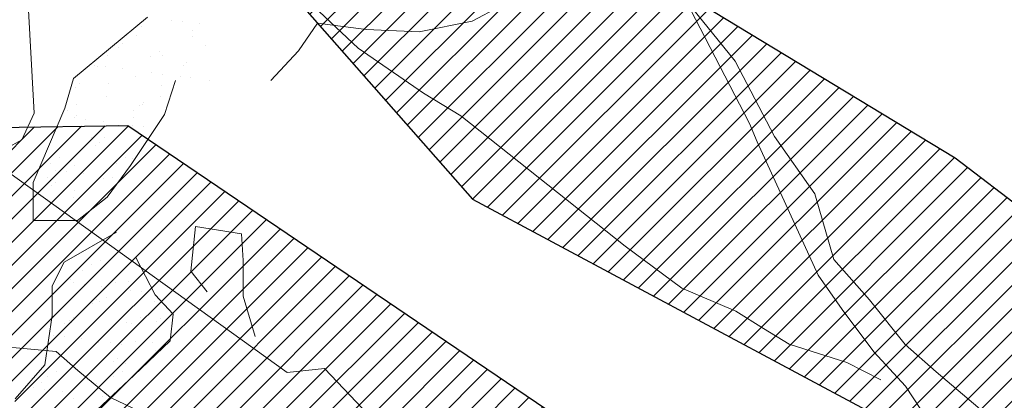
# Model space of a CAD drawing. Units: inches. Extents: x 1986 to 21484, y -1816 to 2016.
# Tile 21 of 85: x 2157.681 to 2166.915, y 1888.377 to 1891.95. Entities that reach past the tile are written whole.
import ezdxf

# ---------------------------------------------------------------- set-up
doc = ezdxf.new("R2010")
doc.units = ezdxf.units.IN
doc.layers.add('L-PLNT', color=84, linetype='Continuous', lineweight=13)
doc.layers.add('vfolhas', color=114, linetype='Continuous', lineweight=5)
doc.layers.add('vfolha2', color=110, linetype='Continuous')
doc.layers.add('vfolhas2', color=102, linetype='Continuous')
pattern_1 = [(45, (-2446.5133113, 50.986076), (-0.004419417382, 0.004419417382), [])]

# ---------------------------------------------------------------- blocks, each defined once
blk = doc.blocks.new('arbusto_PB_verde_grande')
at = {"layer": 'vfolha2'}
h = blk.add_hatch(dxfattribs=at)
h.set_pattern_fill('ANSI31', color=256, scale=0.05, style=0)
h.set_pattern_definition(pattern_1)
h.paths.add_polyline_path([(0.02944, 0.35651), (0.00028, 0.09048), (0.02625, -0.03934), (0.047, 0.06233), (0.06189, 0.09731), (0.09372, 0.26573), (0.09955, 0.43473), (0.08789, 0.61313), (0.0645, 0.72266), (0.04988, 0.6851), (0.0236, 0.51294)])
h.paths.add_polyline_path([(0.30106, 0.43789), (0.14225, 0.24871), (0.26685, 0.30022)])
h.paths.add_polyline_path([(0.37995, 0.22817), (0.23697, 0.15193), (0.18428, 0.09364), (0.11122, 0.04358), (0.02625, -0.03934), (0.28061, 0.04667), (0.36829, 0.07798), (0.46756, 0.11239), (0.61068, 0.19376), (0.71585, 0.27823), (0.55813, 0.25948)])
h.paths.add_polyline_path([(0.56101, -0.29441), (0.72752, -0.32573), (0.59024, -0.2412), (0.42962, -0.15982), (0.02625, -0.03934), (0.14922, -0.14107), (0.18838, -0.16604), (0.41501, -0.24435)])
h.paths.add_polyline_path([(-0.27429, -0.44776), (-0.30352, -0.72628), (-0.23923, -0.64175), (-0.15457, -0.45716), (0.02625, -0.03934), (-0.16328, -0.25376)])
h.paths.add_polyline_path([(-0.51963, -0.24744), (-0.67736, -0.32573), (-0.59558, -0.35072), (-0.40574, -0.32882), (-0.21007, -0.20995), (0.02625, -0.03934), (-0.14874, -0.06595), (-0.31518, -0.09101), (-0.41452, -0.15048)])
h.paths.add_polyline_path([(-0.52546, 0.25007), (-0.70947, 0.24698), (-0.51963, 0.1093), (-0.32979, 0.02167), (-0.07567, -0.0128), (-0.04234, -0.02148), (-0.35024, 0.1312)])
at = {"layer": 'vfolhas'}
h = blk.add_hatch(dxfattribs=at)
h.set_pattern_fill('ANSI31', color=256, scale=0.05, style=0)
h.set_pattern_definition(pattern_1)
h.paths.add_polyline_path([(-0.07279, 0.50669), (-0.18085, 0.65063), (-0.2334, 0.67253), (-0.20712, 0.53176), (-0.10785, 0.25007), (0.02625, -0.03934), (0.00028, 0.09048), (0.00816, 0.16241), (-0.04939, 0.29079)])
h.paths.add_polyline_path([(0.09902, 0.41929), (0.09372, 0.26573), (0.07906, 0.18814), (0.15506, 0.36901), (0.26606, 0.5505), (0.28356, 0.63504), (0.2485, 0.68819), (0.25145, 0.63504), (0.20178, 0.54426)])
h.paths.add_polyline_path([(0.12295, 0.24073), (0.047, 0.06233), (0.02625, -0.03934), (0.11122, 0.04358), (0.18428, 0.09364), (0.27478, 0.19376), (0.3215, 0.25323), (0.44129, 0.38467), (0.47634, 0.57866), (0.41789, 0.45347), (0.28939, 0.30954)])
h.paths.add_polyline_path([(0.58145, -0.03779), (0.70707, 0.01536), (0.78591, 0.04667), (0.74796, 0.06549), (0.62818, 0.08423), (0.52595, 0.09048), (0.39745, 0.04358), (0.02625, -0.03934), (0.25728, -0.03154), (0.43834, -0.0347)])
h.paths.add_polyline_path([(0.52022, -0.03647), (0.43834, -0.0347), (0.25728, -0.03154), (0.02625, -0.03934), (0.17964, -0.08515), (0.53768, -0.13167), (0.69541, -0.15357), (0.78591, -0.07852), (0.70413, -0.10042)])
h.paths.add_polyline_path([(0.27189, -0.21929), (0.14922, -0.14107), (0.02625, -0.03934), (0.15794, -0.31007), (0.29522, -0.42585), (0.41789, -0.49157), (0.56396, -0.56669), (0.5114, -0.48532), (0.39456, -0.34139)])
h.paths.add_polyline_path([(-0.05818, -0.47591), (-0.02312, -0.61984), (0.047, -0.80134), (0.08494, -0.59794), (0.07911, -0.4071), (0.03527, -0.25376), (0.02625, -0.03934), (-0.03773, -0.26001)])
h.paths.add_polyline_path([(-0.24218, 0.14054), (-0.11073, 0.06858), (0.02625, -0.03934), (-0.04235, 0.10871), (-0.21007, 0.23757), (-0.36485, 0.33145), (-0.47874, 0.40341), (-0.54303, 0.46288), (-0.49041, 0.33145), (-0.39408, 0.22192)])
at = {"layer": 'vfolha2'}
for p, q in [((-0.70947, 0.24698), (-0.52546, 0.25007)), ((-0.52546, 0.25007), (-0.35024, 0.1312))]:
    blk.add_line(p, q, dxfattribs=at)
at = {"layer": 'vfolhas2'}
for p, q in [((-0.49041, 0.33145), (-0.39408, 0.22192)), ((-0.21007, 0.23757), (-0.36485, 0.33145)), ((-0.04235, 0.10871), (-0.21007, 0.23757)), ((-0.39408, 0.22192), (-0.24218, 0.14054))]:
    blk.add_line(p, q, dxfattribs=at)
blk = doc.blocks.new('PLANT-SHRUB')
for p, q in [((2157.8167, 1891.0729), (2157.7331, 1892.5683)), ((2163.9242, 1892.1391), (2164.3896, 1891.5609)), ((2164.5252, 1890.9746), (2163.9242, 1892.1391)), ((2160.4349, 1892.0769), (2160.8561, 1891.6818)), ((2162.1841, 1892.075), (2161.9255, 1891.9359)), ((2158.1838, 1891.3968), (2158.8799, 1891.9731)), ((2159.1029, 1891.9467), (2159.1029, 1891.9467)), ((2159.2069, 1891.933), (2159.2069, 1891.933)), ((2161.9255, 1891.9359), (2161.4283, 1891.8365)), ((2158.8222, 1891.886), (2158.8222, 1891.886)), ((2159.2985, 1891.8471), (2159.2985, 1891.8471)), ((2159.3694, 1891.9117), (2159.3694, 1891.9117)), ((2160.4737, 1891.916), (2160.2947, 1891.6576)), ((2160.9311, 1891.8564), (2160.4737, 1891.916)), ((2161.4283, 1891.8365), (2160.9311, 1891.8564)), ((2158.7749, 1891.8029), (2158.7749, 1891.8029)), ((2159.298, 1891.7963), (2159.298, 1891.7963)), ((2158.6115, 1891.6929), (2158.6115, 1891.6929)), ((2158.6484, 1891.7267), (2158.6484, 1891.7267)), ((2158.9952, 1891.6538), (2158.9952, 1891.6538)), ((2159.4229, 1891.7106), (2159.4229, 1891.7106)), ((2160.2947, 1891.6576), (2160.0361, 1891.3794)), ((2160.8561, 1891.6818), (2161.4664, 1891.2609)), ((2158.5047, 1891.6156), (2158.5047, 1891.6156)), ((2158.9109, 1891.6001), (2158.9109, 1891.6001)), ((2159.0159, 1891.618), (2159.0159, 1891.618)), ((2158.3808, 1891.5244), (2158.3808, 1891.5244)), ((2158.4126, 1891.5107), (2158.4126, 1891.5107)), ((2158.4848, 1891.5107), (2158.4848, 1891.5107)), ((2158.6472, 1891.4893), (2158.6472, 1891.4893)), ((2159.2123, 1891.5176), (2159.2123, 1891.5176)), ((2159.2491, 1891.5513), (2159.2491, 1891.5513)), ((2164.3896, 1891.5609), (2164.7593, 1890.8542)), ((2158.1042, 1891.1186), (2158.1838, 1891.3968)), ((2158.7623, 1891.4179), (2158.7623, 1891.4179)), ((2158.9187, 1891.4536), (2158.9187, 1891.4536)), ((2159.0227, 1891.4399), (2159.0227, 1891.4399)), ((2159.1411, 1891.3794), (2159.039, 1891.059)), ((2159.1852, 1891.4185), (2159.1852, 1891.4185)), ((2159.2854, 1891.4112), (2159.2854, 1891.4112)), ((2159.4566, 1891.3828), (2159.4566, 1891.3828)), ((2158.2019, 1891.3176), (2158.2019, 1891.3176)), ((2158.2388, 1891.3514), (2158.2388, 1891.3514)), ((2158.5148, 1891.3478), (2158.5148, 1891.3478)), ((2159.0134, 1891.3353), (2159.0134, 1891.3353)), ((2158.4921, 1891.2305), (2158.4921, 1891.2305)), ((2159.0033, 1891.233), (2159.0033, 1891.233)), ((2161.4664, 1891.2609), (2161.8188, 1891.0462)), ((2160.1908, 1888.6391), (2156.7085, 1891.14)), ((2157.8059, 1890.423), (2158.1042, 1891.1186)), ((2158.1272, 1891.1009), (2158.1272, 1891.1009)), ((2158.2114, 1891.1546), (2158.2114, 1891.1546)), ((2158.7495, 1891.0997), (2158.7495, 1891.0997)), ((2158.8027, 1891.1422), (2158.8027, 1891.1422)), ((2158.8338, 1891.1534), (2158.8338, 1891.1534)), ((2158.8395, 1891.176), (2158.8395, 1891.176)), ((2157.702, 1890.8208), (2157.8167, 1891.0729)), ((2158.1965, 1891.0313), (2158.1965, 1891.0313)), ((2158.21, 1891.0523), (2158.21, 1891.0523)), ((2158.3005, 1891.0176), (2158.3005, 1891.0176)), ((2159.039, 1891.059), (2158.7208, 1890.582)), ((2158.7497, 1891.0329), (2158.7497, 1891.0329)), ((2161.8188, 1891.0462), (2163.3587, 1889.8241)), ((2158.463, 1890.9962), (2158.463, 1890.9962)), ((2158.6038, 1890.96), (2158.6038, 1890.96)), ((2158.7344, 1890.9604), (2158.7344, 1890.9604)), ((2158.8385, 1890.9467), (2158.8385, 1890.9467)), ((2164.5989, 1890.803), (2164.5252, 1890.9746)), ((2158.3534, 1890.8474), (2158.3534, 1890.8474)), ((2158.4795, 1890.8455), (2158.4795, 1890.8455)), ((2164.7593, 1890.8542), (2165.1378, 1890.314)), ((2157.553, 1890.7406), (2157.702, 1890.8208)), ((2158.3931, 1890.7669), (2158.3931, 1890.7669)), ((2158.4299, 1890.8007), (2158.4299, 1890.8007)), ((2165.1697, 1889.5524), (2164.5989, 1890.803)), ((2158.0501, 1890.6541), (2158.0501, 1890.6541)), ((2158.1974, 1890.6673), (2158.1974, 1890.6673)), ((2158.6724, 1890.653), (2158.6724, 1890.653)), ((2158.7371, 1890.6478), (2158.7371, 1890.6478)), ((2157.9658, 1890.6005), (2157.9658, 1890.6005)), ((2158.1942, 1890.5847), (2158.1942, 1890.5847)), ((2158.7208, 1890.582), (2158.502, 1890.2839)), ((2158.5881, 1890.5993), (2158.5881, 1890.5993)), ((2157.9438, 1890.4671), (2157.9438, 1890.4671)), ((2158.0123, 1890.5381), (2158.0123, 1890.5381)), ((2158.1163, 1890.5244), (2158.1163, 1890.5244)), ((2158.2788, 1890.503), (2158.2788, 1890.503)), ((2158.4669, 1890.4604), (2158.4669, 1890.4604)), ((2158.5502, 1890.4673), (2158.5502, 1890.4673)), ((2157.8059, 1890.0653), (2157.8059, 1890.423)), ((2157.9835, 1890.3916), (2157.9835, 1890.3916)), ((2158.0203, 1890.4253), (2158.0203, 1890.4253)), ((2158.1848, 1890.2822), (2158.1848, 1890.2822)), ((2158.192, 1890.347), (2158.192, 1890.347)), ((2158.502, 1890.2839), (2158.2236, 1890.0653)), ((2165.1378, 1890.314), (2165.3178, 1889.6975)), ((2158.2236, 1890.0653), (2157.8059, 1890.0653)), ((2159.2867, 1889.5907), (2159.3286, 1890.0097)), ((2159.3286, 1890.0097), (2159.7619, 1889.9399)), ((2158.0985, 1889.6745), (2158.5877, 1889.9538)), ((2158.5877, 1889.9538), (2158.5877, 1889.9538)), ((2159.7619, 1889.9399), (2159.7759, 1889.6884)), ((2163.3587, 1889.8241), (2163.8916, 1889.429)), ((2158.7695, 1889.7164), (2158.9512, 1889.3672)), ((2157.9866, 1889.451), (2158.0985, 1889.6745)), ((2158.3496, 1889.6522), (2158.3496, 1889.6522)), ((2158.4418, 1889.6903), (2158.4418, 1889.6903)), ((2159.7759, 1889.6884), (2159.7759, 1889.3532)), ((2165.3178, 1889.6975), (2165.652, 1889.3207)), ((2158.2653, 1889.5985), (2158.2653, 1889.5985)), ((2159.4404, 1889.3951), (2159.2867, 1889.5907)), ((2165.3932, 1889.2298), (2165.1697, 1889.5524)), ((2157.9866, 1889.1716), (2157.9866, 1889.451)), ((2158.1596, 1889.5121), (2158.1596, 1889.5121)), ((2158.1817, 1889.481), (2158.1817, 1889.481)), ((2158.2857, 1889.4673), (2158.2857, 1889.4673)), ((2158.4482, 1889.4459), (2158.4482, 1889.4459)), ((2158.5765, 1889.4832), (2158.5765, 1889.4832)), ((2158.6994, 1889.4927), (2158.6994, 1889.4927)), ((2158.4916, 1889.3451), (2158.4916, 1889.3451)), ((2158.7196, 1889.4102), (2158.7196, 1889.4102)), ((2158.8236, 1889.3965), (2158.8236, 1889.3965)), ((2158.9512, 1889.3672), (2159.1189, 1889.1856)), ((2159.7759, 1889.3532), (2159.8877, 1888.9761)), ((2163.8916, 1889.429), (2164.3988, 1889.2143)), ((2158.3658, 1889.2902), (2158.3658, 1889.2902)), ((2158.4026, 1889.3239), (2158.4026, 1889.3239)), ((2158.4292, 1889.3053), (2158.4292, 1889.3053)), ((2158.9404, 1889.3078), (2158.9404, 1889.3078)), ((2165.652, 1889.3207), (2165.9862, 1888.9011)), ((2157.9168, 1888.7107), (2157.9866, 1889.1716)), ((2159.1189, 1889.1856), (2159.091, 1888.9342)), ((2164.3988, 1889.2143), (2164.6567, 1889.0511)), ((2165.3932, 1889.2298), (2165.3932, 1889.2298)), ((2165.6912, 1888.8328), (2165.3932, 1889.2298)), ((2158.1039, 1889.0981), (2158.1039, 1889.0981)), ((2158.1471, 1889.1271), (2158.1471, 1889.1271)), ((2158.1669, 1889.1079), (2158.1669, 1889.1079)), ((2158.1882, 1889.1518), (2158.1882, 1889.1518)), ((2158.6868, 1889.1076), (2158.6868, 1889.1076)), ((2158.7262, 1889.097), (2158.7262, 1889.097)), ((2158.8105, 1889.1507), (2158.8105, 1889.1507)), ((2158.9665, 1889.1148), (2158.9665, 1889.1148)), ((2159.0033, 1889.1485), (2159.0033, 1889.1485)), ((2157.9974, 1888.9879), (2157.9974, 1888.9879)), ((2164.6567, 1889.0511), (2164.8973, 1888.9051)), ((2158.0239, 1888.8339), (2157.475, 1888.8845)), ((2157.9562, 1888.9149), (2157.9562, 1888.9149)), ((2157.993, 1888.9486), (2157.993, 1888.9486)), ((2158.1015, 1888.9742), (2158.1015, 1888.9742)), ((2158.2639, 1888.9528), (2158.2639, 1888.9528)), ((2158.4166, 1888.9203), (2158.4166, 1888.9203)), ((2158.5354, 1888.917), (2158.5354, 1888.917)), ((2158.6394, 1888.9033), (2158.6394, 1888.9033)), ((2159.091, 1888.9342), (2158.7555, 1888.6129)), ((2158.7676, 1888.9325), (2158.7676, 1888.9325)), ((2158.9278, 1888.9227), (2158.9278, 1888.9227)), ((2164.8973, 1888.9051), (2165.4389, 1888.7333)), ((2165.9862, 1888.9011), (2166.2776, 1888.6442)), ((2158.2267, 1888.6574), (2158.0239, 1888.8339)), ((2158.3302, 1888.8447), (2158.3302, 1888.8447)), ((2158.8018, 1888.882), (2158.8018, 1888.882)), ((2158.9525, 1888.8435), (2158.9525, 1888.8435)), ((2165.9892, 1888.5102), (2165.6912, 1888.8328)), ((2157.6372, 1888.3894), (2157.9168, 1888.7107)), ((2158.1345, 1888.742), (2158.1345, 1888.742)), ((2158.5569, 1888.7395), (2158.5569, 1888.7395)), ((2158.5938, 1888.7732), (2158.5938, 1888.7732)), ((2158.6742, 1888.7226), (2158.6742, 1888.7226)), ((2165.4389, 1888.7333), (2165.7569, 1888.5701)), ((2158.0268, 1888.6514), (2158.0268, 1888.6514)), ((2158.5318, 1888.4034), (2158.2267, 1888.6574)), ((2158.7555, 1888.6129), (2158.3082, 1888.1939)), ((2158.6491, 1888.6503), (2158.6491, 1888.6503)), ((2160.5404, 1888.674), (2160.1908, 1888.6391)), ((2161.292, 1887.888), (2160.5404, 1888.674)), ((2166.2776, 1888.6442), (2166.8518, 1888.1561)), ((2157.8809, 1888.5419), (2157.8809, 1888.5419)), ((2157.9425, 1888.5977), (2157.9425, 1888.5977)), ((2158.358, 1888.5572), (2158.358, 1888.5572)), ((2158.404, 1888.5352), (2158.404, 1888.5352)), ((2158.5648, 1888.5966), (2158.5648, 1888.5966)), ((2157.8132, 1888.4947), (2157.8132, 1888.4947)), ((2157.9172, 1888.481), (2157.9172, 1888.481)), ((2158.0797, 1888.4596), (2158.0797, 1888.4596)), ((2158.3511, 1888.4239), (2158.3511, 1888.4239)), ((2166.3617, 1887.9395), (2165.9892, 1888.5102)), ((2158.1842, 1888.3979), (2158.1842, 1888.3979)), ((2158.4551, 1888.4102), (2158.4551, 1888.4102)), ((2159.4328, 1887.9763), (2158.5318, 1888.4034))]:
    blk.add_line(p, q)

msp = doc.modelspace()

# ---------------------------------------------------------------- block references
at = {"layer": 'L-PLNT'}
msp.add_blockref('PLANT-SHRUB', (0, 0), dxfattribs=at)
at = {"layer": 'L-PLNT', "xscale": 24.60366729364114, "yscale": 24.60366729364114, "zscale": 24.60366729364114}
msp.add_blockref('arbusto_PB_verde_grande', (2171.6234, 1884.8051), dxfattribs=at)

doc.saveas('drawing.dxf')
